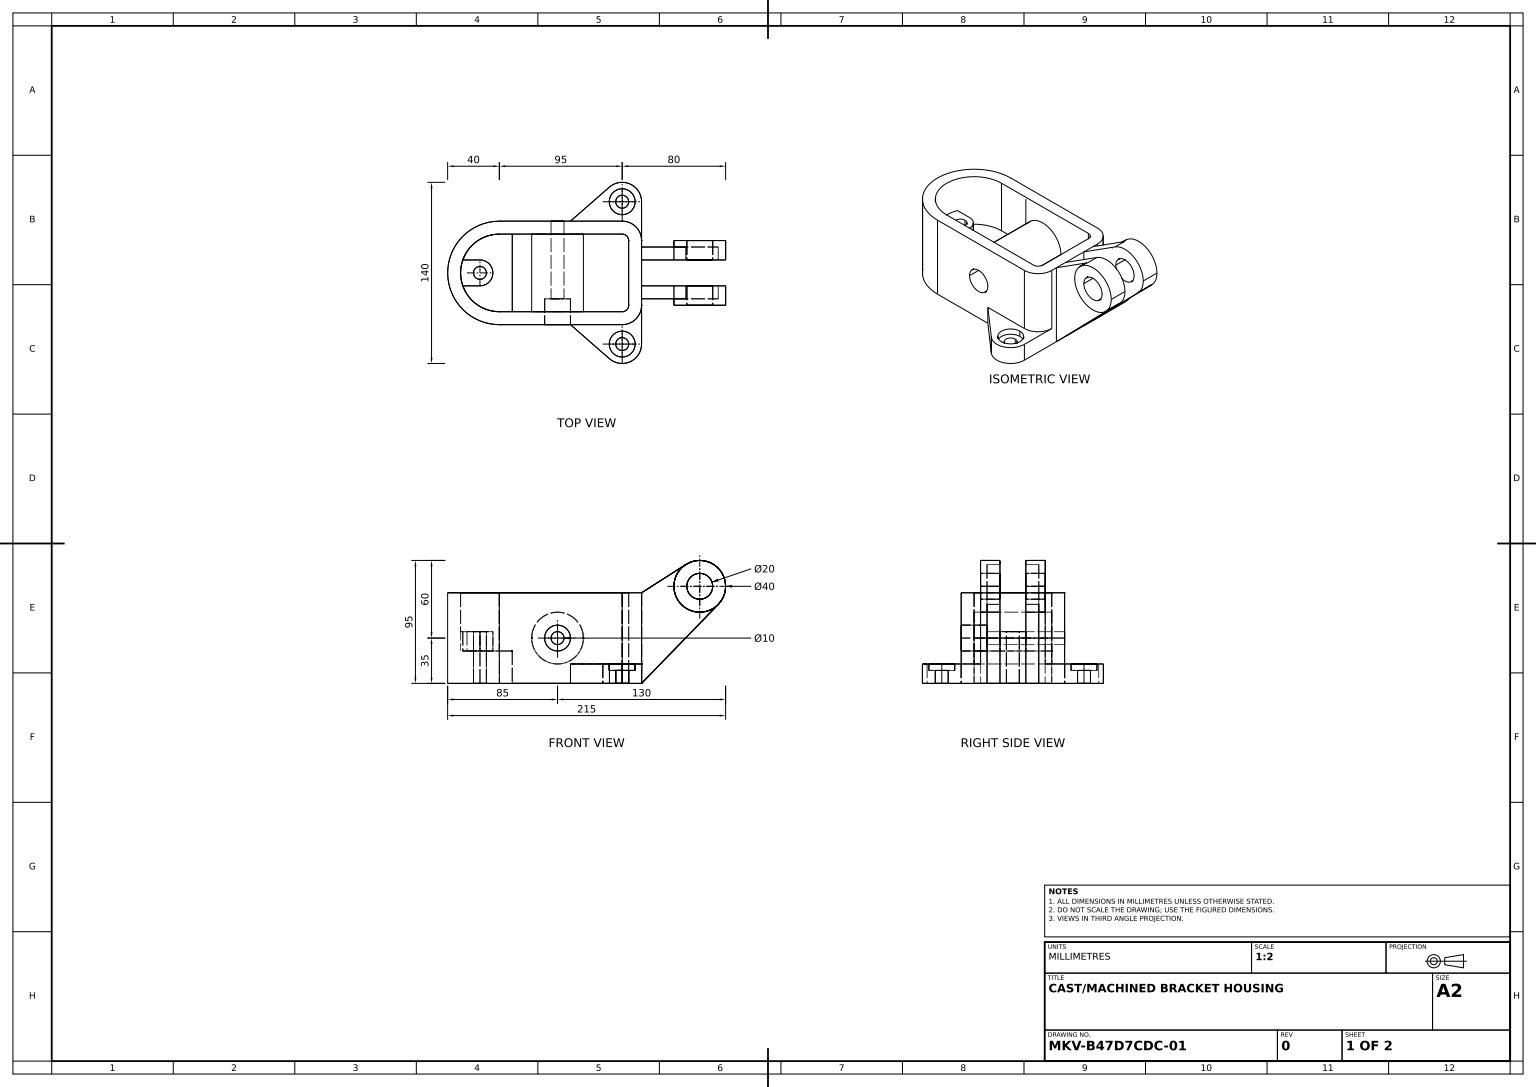
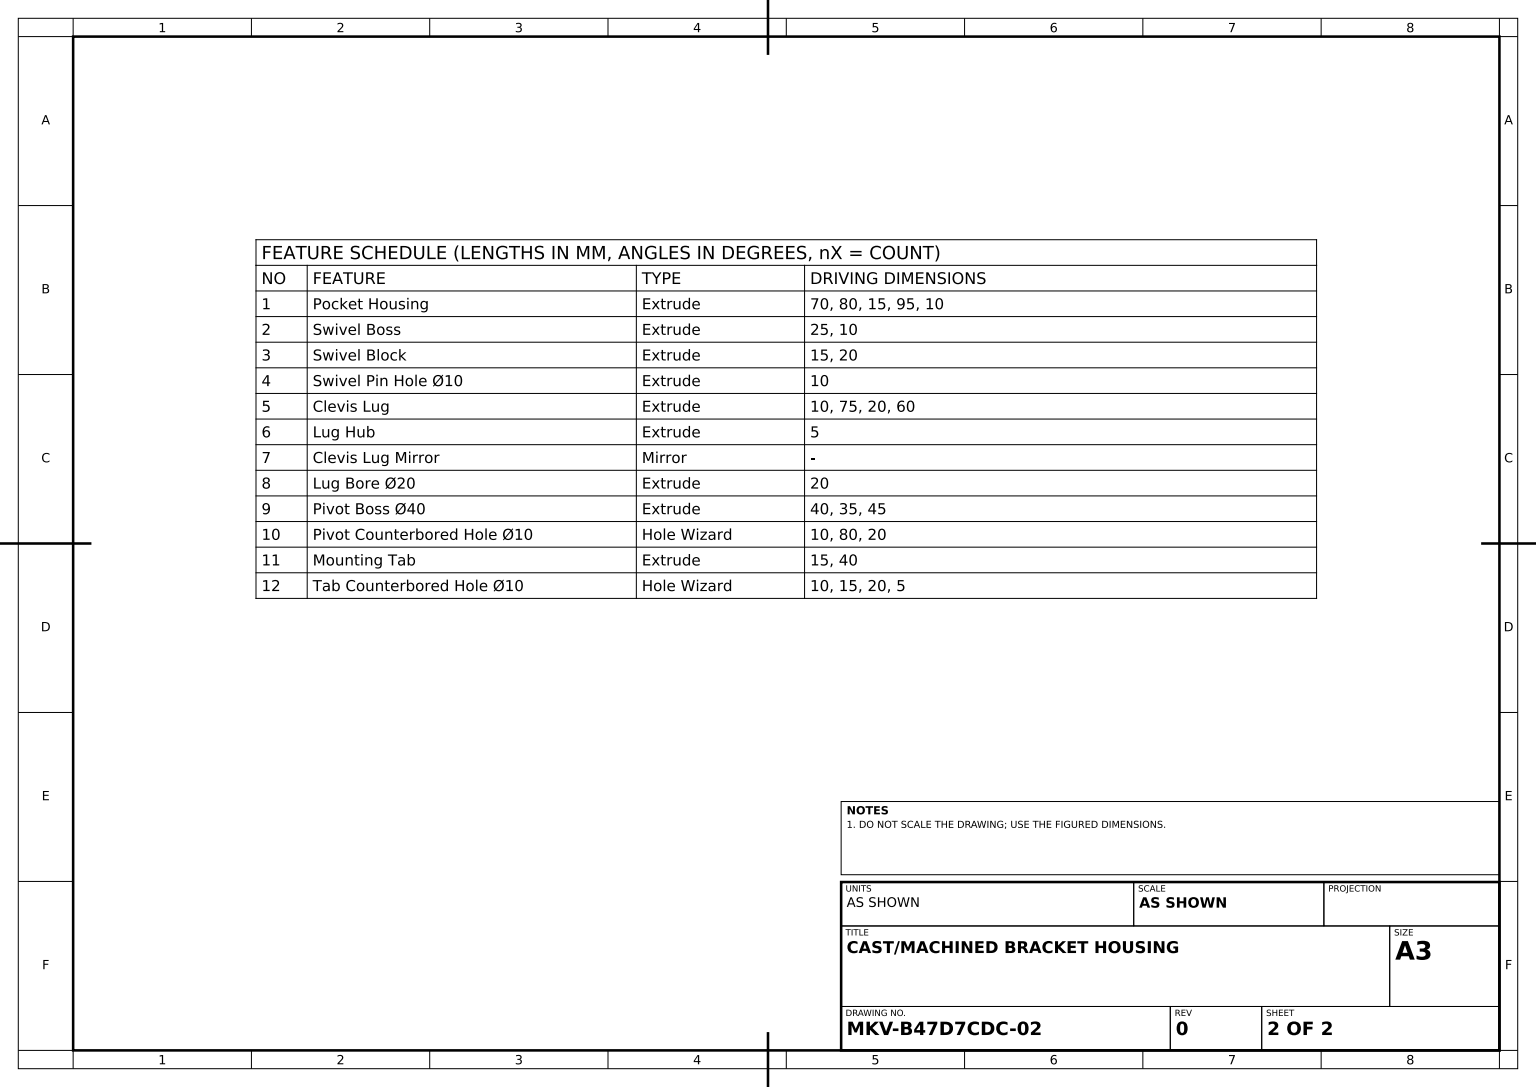
from build123d import *

# Parameters (mm, degrees)
POCKET_HOUSING_DEPTH                   = 70
SWIVEL_BOSS_DEPTH                      = 25
SWIVEL_BLOCK_DEPTH                     = 15
SWIVEL_PIN_HOLE_SKETCH_R               = 5
SWIVEL_PIN_HOLE_10_DEPTH               = 161.312195419
CLEVIS_START                           = 10
CLEVIS_LUG_DEPTH                       = 10
LUG_HUB_SKETCH_R                       = 20
LUG_HUB_DEPTH                          = 5
LUG_BORE_20_DEPTH                      = 190.076704012
LUG_BORE_20_DEPTH_BACK                 = 190.076704012
LUG_BORE_SKETCH_R                      = 10
PIVOT_BOSS_SKETCH_R                    = 20
PIVOT_BOSS_40_DEPTH                    = 80
PIVOT_COUNTERBORED_HOLE_10_D           = 10
PIVOT_COUNTERBORED_HOLE_10_CBORE_D     = 20
PIVOT_COUNTERBORED_HOLE_10_CBORE_DEPTH = 20
MOUNTING_TAB_DEPTH                     = 15
TAB_COUNTERBORED_HOLE_10_D             = 10
TAB_COUNTERBORED_HOLE_10_CBORE_D       = 20
TAB_COUNTERBORED_HOLE_10_CBORE_DEPTH   = 5


with BuildPart() as part:
    # Pocket Housing Sketch → Pocket Housing (new body)
    with BuildSketch(Plane(origin=(0, 0, 0), x_dir=(1, 0, 0), z_dir=(0, 1, 0))):
        with BuildLine():
            Line((0, 0), (0, 25))
            ThreePointArc((0, 25), (-4.393398282, 35.606601718), (-15, 40))
            Line((-15, 40), (-110, 40))
            ThreePointArc((-110, 40), (-150, 0), (-110, -40))
            Line((-110, -40), (-15, -40))
            ThreePointArc((-15, -40), (-4.393398282, -35.606601718), (0, -25))
            Line((0, -25), (0, 0))
        make_face()
        with BuildLine():
            Line((-15, 30), (-110, 30))
            ThreePointArc((-110, 30), (-140, 0), (-110, -30))
            Line((-110, -30), (-15, -30))
            ThreePointArc((-15, -30), (-11.464466094, -28.535533906), (-10, -25))
            Line((-10, -25), (-10, 0))
            Line((-10, 0), (-10, 25))
            ThreePointArc((-10, 25), (-11.464466094, 28.535533906), (-15, 30))
        make_face(mode=Mode.SUBTRACT)
    extrude(amount=POCKET_HOUSING_DEPTH)

    # Swivel Boss Sketch → Swivel Boss (add)
    with BuildSketch(Plane(origin=(0, 0, 0), x_dir=(1, 0, 0), z_dir=(0, 1, 0))):
        with BuildLine():
            Line((-100, 30), (-100, -30))
            Line((-100, -30), (-110, -30))
            ThreePointArc((-110, -30), (-140, 0), (-110, 30))
            Line((-110, 30), (-100, 30))
        make_face()
    extrude(amount=SWIVEL_BOSS_DEPTH)

    # Swivel Block Sketch → Swivel Block (add)
    with BuildSketch(Plane(origin=(0, 25, 0), x_dir=(1, 0, 0), z_dir=(0, 1, 0))):
        with BuildLine():
            Line((-125, -10), (-138.284271247, -10))
            ThreePointArc((-138.284271247, -10), (-140, 0), (-138.284271247, 10))
            Line((-138.284271247, 10), (-125, 10))
            ThreePointArc((-125, 10), (-115, 0), (-125, -10))
        make_face()
    extrude(amount=SWIVEL_BLOCK_DEPTH)

    # Swivel Pin Hole Sketch → Swivel Pin Hole Ø10 (cut, through all)
    with BuildSketch(Plane(origin=(0, 40, 0), x_dir=(1, 0, 0), z_dir=(0, 1, 0))):
        with Locations(Location((-125, 0, 0), (0, 0, 270))):
            Circle(SWIVEL_PIN_HOLE_SKETCH_R)
    extrude(amount=-SWIVEL_PIN_HOLE_10_DEPTH, mode=Mode.SUBTRACT)

    # Clevis Lug Sketch → Clevis Lug (add)
    with BuildSketch(Plane.XY.offset(CLEVIS_START)):
        with BuildLine():
            Line((0, 70), (34.238039414, 91.857645278))
            ThreePointArc((34.238039414, 91.857645278), (60.501975118, 87.636802105), (59.342535653, 61.061145275))
            Line((59.342535653, 61.061145275), (0, 0))
            Line((0, 0), (0, 70))
        make_face()
    clevis_lug = extrude(amount=CLEVIS_LUG_DEPTH)

    # Lug Hub Sketch → Lug Hub (add)
    with BuildSketch(Plane.XY.offset(20)):
        with Locations(Location((45, 75, 0), (0, 0, 122.554257086))):
            Circle(LUG_HUB_SKETCH_R)
    lug_hub = extrude(amount=LUG_HUB_DEPTH)

    # Clevis Lug Mirror: Clevis Lug, Lug Hub across plane
    add(clevis_lug.mirror(Plane.XY))
    add(lug_hub.mirror(Plane.XY))

    # Lug Bore Sketch → Lug Bore Ø20 (cut, two sides: drawn at the far end of the back side and taken through both)
    with BuildSketch(Plane.XY.offset(25).offset(-LUG_BORE_20_DEPTH_BACK)):
        with Locations(Location((45, 75, 0), (0, 0, 180))):
            Circle(LUG_BORE_SKETCH_R)
    extrude(amount=LUG_BORE_20_DEPTH + LUG_BORE_20_DEPTH_BACK, mode=Mode.SUBTRACT)

    # Pivot Boss Sketch → Pivot Boss Ø40 (add)
    with BuildSketch(Plane.XY.offset(40)):
        with Locations((-65, 35)):
            Circle(PIVOT_BOSS_SKETCH_R)
    extrude(amount=-PIVOT_BOSS_40_DEPTH)

    # Pivot Counterbored Hole Ø10 (through all)
    with Locations(Plane(origin=(-65, 35, 40), x_dir=(1, 0, 0), z_dir=(0, 0, 1))):
        with Locations((0, 0)):
            CounterBoreHole(PIVOT_COUNTERBORED_HOLE_10_D / 2, PIVOT_COUNTERBORED_HOLE_10_CBORE_D / 2, PIVOT_COUNTERBORED_HOLE_10_CBORE_DEPTH)

    # Mounting Tab Sketch → Mounting Tab (add)
    with BuildSketch(Plane(origin=(0, 0, 0), x_dir=(1, 0, 0), z_dir=(0, 1, 0))):
        with BuildLine():
            Line((0, 25), (0, 55))
            ThreePointArc((0, 55), (-8.792955835, 68.655497162), (-24.863013699, 66.301369863))
            Line((-24.863013699, 66.301369863), (-55, 40))
            Line((-55, 40), (-15, 40))
            ThreePointArc((-15, 40), (-4.393398282, 35.606601718), (0, 25))
        make_face()
        with BuildLine():
            Line((0, -25), (0, -55))
            ThreePointArc((0, -55), (-8.792955835, -68.655497162), (-24.863013699, -66.301369863))
            Line((-24.863013699, -66.301369863), (-55, -40))
            Line((-55, -40), (-15, -40))
            ThreePointArc((-15, -40), (-4.393398282, -35.606601718), (0, -25))
        make_face()
    extrude(amount=MOUNTING_TAB_DEPTH)

    # Tab Counterbored Hole Ø10 (through all)
    with Locations(Plane(origin=(-15, 15, 55), x_dir=(0, 0, 1), z_dir=(0, 1, 0))):
        with Locations((0, 0), (-110, 0)):
            CounterBoreHole(TAB_COUNTERBORED_HOLE_10_D / 2, TAB_COUNTERBORED_HOLE_10_CBORE_D / 2, TAB_COUNTERBORED_HOLE_10_CBORE_DEPTH)


solid = part.part
